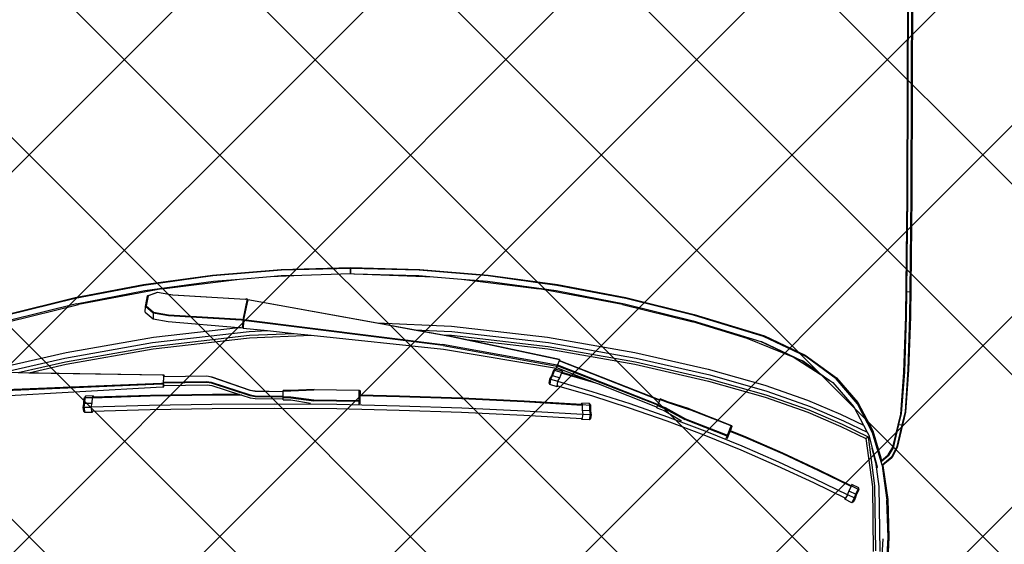
# Model space of a CAD drawing. Units: inches. Extents: x 2167 to 2589, y 1680 to 2489.
# Tile 21 of 38: x 2269 to 2306, y 1796 to 1815. Entities that reach past the tile are written whole.
import ezdxf

# ---------------------------------------------------------------- set-up
doc = ezdxf.new("R2010")
doc.units = ezdxf.units.IN
doc.header["$MEASUREMENT"] = 0
doc.layers.get('0').update_dxf_attribs({"color": 250})
for name, color, linetype, lineweight in [('A-ANNO-DIMS', 2, 'Continuous', 18), ('C-PRKG-VEHS', 8, 'Continuous', 13), ('L-PVMT-PATT', 252, 'Continuous', 13)]:
    doc.layers.add(name, color=color, linetype=linetype, lineweight=lineweight)
doc.layers.add('Edges', color=250, linetype='Continuous')
doc.styles.get("Standard").update_dxf_attribs({"font": 'arial.ttf'})
doc.dimstyles.get("Standard").update_dxf_attribs({"dimtxt": 7, "dimasz": 0.18, "dimexe": 0.18, "dimexo": 0.0625, "dimgap": 0.09, "dimtad": 0, "dimtih": 1, "dimtoh": 1, "dimdec": 1, "dimzin": 0, "dimdsep": 46, "dimlunit": 3, "dimtxsty": 'Standard', "dimcen": 0.09, "dimadec": 0, "dimazin": 0, "dimtfac": 1, "dimtdec": 1, "dimtofl": 0, "dimtmove": 0, "dimatfit": 3, "dimfxl": 1, "dimtolj": 1, "dimtzin": 0, "dimarcsym": 0})

# ---------------------------------------------------------------- blocks, each defined once
blk = doc.blocks.new('Nissan Qashqai pl')
at = {"layer": 'Edges'}
for p, q in [((8.0273, 12.6485), (7.9014, 12.6487)), ((8.0275, 12.6493), (7.902, 12.6495)), ((7.9036, 12.6534), (8.0275, 12.6533)), ((7.904, 12.6547), (8.0276, 12.6545)), ((8.1753, 12.6479), (8.0273, 12.6485)), ((8.0275, 12.6533), (8.1755, 12.6527)), ((8.1754, 12.6487), (8.0275, 12.6493)), ((8.0276, 12.6545), (8.1753, 12.6539)), ((8.1753, 12.6539), (8.3324, 12.6521)), ((8.3318, 12.6462), (8.1753, 12.6479)), ((8.3002, 12.6474), (8.1754, 12.6487)), ((8.1755, 12.6527), (8.3005, 12.6514)), ((8.3005, 12.6514), (8.3002, 12.6474)), ((8.332, 12.6471), (8.3002, 12.6474)), ((8.3005, 12.6514), (8.3324, 12.651)), ((8.4049, 12.6437), (8.3318, 12.6462)), ((8.4042, 12.6447), (8.332, 12.6471)), ((8.3324, 12.6521), (8.4022, 12.6498)), ((8.3324, 12.651), (8.4014, 12.6488)), ((8.4014, 12.6488), (8.4559, 12.6451)), ((8.4022, 12.6498), (8.4571, 12.6459)), ((8.4559, 12.6451), (8.4736, 12.6409)), ((8.4571, 12.6459), (8.5029, 12.635)), ((8.4588, 12.6405), (8.4042, 12.6447)), ((8.4595, 12.6395), (8.4049, 12.6437)), ((8.4729, 12.6372), (8.4588, 12.6405)), ((8.5025, 12.6293), (8.4595, 12.6395)), ((8.4729, 12.6372), (8.4736, 12.6409)), ((8.5032, 12.6301), (8.4729, 12.6372)), ((8.4736, 12.6409), (8.5018, 12.6344)), ((8.5018, 12.6344), (8.5155, 12.6274)), ((8.5029, 12.635), (8.5163, 12.6279)), ((8.5125, 12.6231), (8.5025, 12.6293)), ((8.5132, 12.624), (8.5032, 12.6301)), ((8.5177, 12.617), (8.5125, 12.6231)), ((8.5132, 12.624), (8.5216, 12.6139)), ((8.5155, 12.6274), (8.5258, 12.6151)), ((8.5163, 12.6279), (8.5237, 12.6189)), ((8.5294, 12.6167), (8.5706, 12.6226)), ((8.5304, 12.6157), (8.5715, 12.6215)), ((8.5706, 12.6226), (8.6197, 12.6241)), ((8.6203, 12.6229), (8.5715, 12.6215)), ((8.6197, 12.6241), (8.6683, 12.6215)), ((8.6203, 12.6229), (8.6204, 12.6229)), ((8.6721, 12.6201), (8.6204, 12.6229)), ((8.4814, 12.6029), (8.5166, 12.6135)), ((8.5216, 12.6139), (8.4838, 12.6027)), ((8.5039, 12.6023), (8.528, 12.6088)), ((8.5216, 12.6068), (8.5039, 12.6023)), ((8.5166, 12.6135), (8.5197, 12.6145)), ((8.5197, 12.6145), (8.5177, 12.617)), ((8.5197, 12.6145), (8.5216, 12.6139)), ((8.5258, 12.6151), (8.5216, 12.6139)), ((8.5216, 12.6068), (8.5538, 12.6111)), ((8.5301, 12.609), (8.5216, 12.6068)), ((8.5237, 12.6189), (8.5259, 12.6162)), ((8.5259, 12.6162), (8.5258, 12.6151)), ((8.5258, 12.6151), (8.5304, 12.6157)), ((8.5259, 12.6162), (8.5294, 12.6167)), ((8.5304, 12.6157), (8.5304, 12.6157)), ((8.5531, 12.6055), (8.6375, 12.6066)), ((8.5538, 12.6111), (8.6387, 12.6123)), ((8.622, 12.6161), (8.6699, 12.6132)), ((8.4444, 12.5834), (8.4814, 12.6029)), ((8.4838, 12.6027), (8.4462, 12.5833)), ((8.468, 12.5648), (8.4831, 12.5957)), ((8.4725, 12.563), (8.4889, 12.5969)), ((8.4737, 12.5908), (8.4831, 12.5957)), ((8.4756, 12.5615), (8.4914, 12.5942)), ((8.4831, 12.5957), (8.4867, 12.5977)), ((8.4867, 12.5977), (8.5039, 12.6023)), ((8.4889, 12.5969), (8.5531, 12.6055)), ((8.4914, 12.5942), (8.4889, 12.5969)), ((8.4914, 12.5942), (8.5544, 12.6026)), ((8.5544, 12.6026), (8.6386, 12.6037)), ((8.4122, 12.5558), (8.4444, 12.5834)), ((8.4462, 12.5833), (8.4134, 12.5554)), ((8.4499, 12.5782), (8.4737, 12.5908)), ((8.4594, 12.5611), (8.4737, 12.5908)), ((8.5554, 12.5847), (8.551, 12.5757)), ((8.5529, 12.5751), (8.5572, 12.5841)), ((8.5574, 12.5849), (8.5554, 12.5847)), ((8.5572, 12.5841), (8.5554, 12.5847)), ((8.5639, 12.581), (8.5572, 12.5841)), ((8.5574, 12.5849), (8.5584, 12.5846)), ((8.5582, 12.5845), (8.5574, 12.5849)), ((8.5584, 12.5846), (8.5649, 12.5816)), ((8.5595, 12.572), (8.5639, 12.581)), ((8.5687, 12.5791), (8.5639, 12.581)), ((8.5649, 12.5816), (8.5693, 12.5799)), ((8.4183, 12.5508), (8.4499, 12.5782)), ((8.5527, 12.5749), (8.5323, 12.5332)), ((8.5537, 12.5747), (8.5332, 12.5329)), ((8.5647, 12.57), (8.5441, 12.5279)), ((8.5527, 12.5749), (8.551, 12.5757)), ((8.551, 12.5757), (8.5528, 12.5751)), ((8.5528, 12.5751), (8.5527, 12.5749)), ((8.5528, 12.5751), (8.5529, 12.5751)), ((8.5529, 12.5751), (8.5537, 12.5747)), ((8.5537, 12.5747), (8.5595, 12.572)), ((8.5595, 12.572), (8.5644, 12.5701)), ((8.5644, 12.5701), (8.5687, 12.5791)), ((8.5644, 12.5701), (8.5647, 12.57)), ((8.5647, 12.57), (8.5692, 12.5675)), ((8.5687, 12.5791), (8.5693, 12.5799)), ((8.5749, 12.5757), (8.5687, 12.5791)), ((8.5693, 12.5799), (8.5739, 12.5774)), ((8.5749, 12.5757), (8.5705, 12.5668)), ((8.5739, 12.5774), (8.5749, 12.5757)), ((8.3826, 12.5151), (8.4122, 12.5558)), ((8.4134, 12.5554), (8.3844, 12.5157)), ((8.4411, 12.5178), (8.4594, 12.5611)), ((8.4493, 12.5212), (8.468, 12.5648)), ((8.454, 12.5196), (8.4725, 12.563)), ((8.4571, 12.5184), (8.4756, 12.5615)), ((8.5487, 12.5256), (8.5692, 12.5674)), ((8.5692, 12.5674), (8.5692, 12.5675)), ((8.5692, 12.5675), (8.5705, 12.5668)), ((8.5705, 12.5668), (8.5692, 12.5674)), ((8.4154, 12.5468), (8.3852, 12.4994)), ((8.3901, 12.5113), (8.4154, 12.5468)), ((8.4011, 12.5269), (8.4154, 12.5468)), ((8.4156, 12.547), (8.4154, 12.5468)), ((8.4156, 12.547), (8.4183, 12.5508)), ((8.5323, 12.5332), (8.5103, 12.4859)), ((8.5332, 12.5329), (8.5112, 12.4856)), ((8.4011, 12.5269), (8.3901, 12.5113)), ((8.3904, 12.512), (8.4011, 12.5269)), ((8.4217, 12.4622), (8.4411, 12.5178)), ((8.4296, 12.4651), (8.4493, 12.5212)), ((8.4343, 12.4637), (8.454, 12.5196)), ((8.4375, 12.4627), (8.4571, 12.5184)), ((8.5441, 12.5279), (8.5222, 12.4807)), ((8.5269, 12.4785), (8.5487, 12.5256)), ((8.3573, 12.4618), (8.3826, 12.5151)), ((8.3844, 12.5157), (8.3582, 12.4606)), ((8.3646, 12.4572), (8.39, 12.5111)), ((8.3648, 12.4579), (8.39, 12.5111)), ((8.39, 12.5111), (8.3852, 12.4994)), ((8.39, 12.5111), (8.3901, 12.5113)), ((8.3901, 12.5113), (8.3904, 12.512)), ((8.3852, 12.4994), (8.3608, 12.4393)), ((8.5103, 12.4859), (8.4895, 12.4381)), ((8.5112, 12.4856), (8.4904, 12.4377)), ((8.5222, 12.4807), (8.5014, 12.4329)), ((8.5062, 12.431), (8.5269, 12.4785)), ((8.3296, 12.3703), (8.3573, 12.4618)), ((8.3582, 12.4606), (8.3311, 12.3708)), ((8.3377, 12.3689), (8.3646, 12.4572)), ((8.3646, 12.4572), (8.3648, 12.4579)), ((8.3648, 12.4579), (8.3648, 12.4579)), ((8.4009, 12.3883), (8.4217, 12.4622)), ((8.4084, 12.3907), (8.4296, 12.4651)), ((8.4133, 12.3896), (8.4343, 12.4637)), ((8.4165, 12.3888), (8.4375, 12.4627)), ((8.3608, 12.4393), (8.3392, 12.3684)), ((8.3608, 12.4393), (8.3608, 12.4393)), ((8.4895, 12.4381), (8.4811, 12.4174)), ((8.5014, 12.4329), (8.4817, 12.3847)), ((8.4904, 12.4377), (8.482, 12.4171)), ((8.4866, 12.3829), (8.5062, 12.431)), ((8.4526, 12.3639), (8.4742, 12.4188)), ((8.4747, 12.4185), (8.4532, 12.3636)), ((8.4742, 12.4188), (8.4754, 12.4193)), ((8.4747, 12.4185), (8.4742, 12.4188)), ((8.4754, 12.4193), (8.4747, 12.4185)), ((8.4869, 12.4136), (8.4747, 12.4185)), ((8.4754, 12.4193), (8.4876, 12.4144)), ((8.4791, 12.4183), (8.4754, 12.4193)), ((8.4811, 12.4174), (8.4791, 12.4183)), ((8.482, 12.4171), (8.4811, 12.4174)), ((8.4912, 12.4133), (8.482, 12.4171)), ((8.4869, 12.4136), (8.4876, 12.4144)), ((8.4876, 12.4144), (8.4912, 12.4133)), ((8.4876, 12.4144), (8.4881, 12.4131)), ((8.4654, 12.3587), (8.4869, 12.4136)), ((8.4881, 12.4131), (8.4666, 12.3582)), ((8.4881, 12.4131), (8.4869, 12.4136)), ((8.4914, 12.4121), (8.4881, 12.4131)), ((8.4913, 12.4133), (8.4912, 12.4133)), ((8.4913, 12.4132), (8.4913, 12.4133)), ((8.3792, 12.2926), (8.4009, 12.3883)), ((8.3864, 12.2945), (8.4084, 12.3907)), ((8.3913, 12.2935), (8.4133, 12.3896)), ((8.3945, 12.2929), (8.4165, 12.3888)), ((8.4817, 12.3847), (8.4633, 12.3359)), ((8.4683, 12.3345), (8.4866, 12.3829)), ((8.3076, 12.281), (8.3296, 12.3703)), ((8.3311, 12.3708), (8.3089, 12.2811)), ((8.3157, 12.2795), (8.3377, 12.3689)), ((8.3166, 12.2767), (8.3392, 12.3684)), ((8.4526, 12.3639), (8.4434, 12.3353)), ((8.4439, 12.335), (8.4532, 12.3636)), ((8.4509, 12.3322), (8.4654, 12.3587)), ((8.4521, 12.3317), (8.4666, 12.3582)), ((8.4547, 12.3309), (8.4682, 12.3538)), ((8.3894, 12.1944), (8.4409, 12.3255)), ((8.4415, 12.3252), (8.3899, 12.1941)), ((8.4434, 12.3353), (8.4397, 12.326)), ((8.4403, 12.3257), (8.4397, 12.326)), ((8.4403, 12.3257), (8.4439, 12.335)), ((8.4409, 12.3255), (8.4403, 12.3257)), ((8.4415, 12.3252), (8.4409, 12.3255)), ((8.4467, 12.3231), (8.4415, 12.3252)), ((8.4633, 12.3359), (8.4461, 12.2868)), ((8.4472, 12.3229), (8.4509, 12.3322)), ((8.4484, 12.3224), (8.4521, 12.3317)), ((8.4511, 12.3216), (8.4547, 12.3309)), ((8.4512, 12.2856), (8.4683, 12.3345)), ((8.3951, 12.192), (8.4467, 12.3231)), ((8.4479, 12.3226), (8.3963, 12.1915)), ((8.4209, 12.2475), (8.4502, 12.3219)), ((8.4472, 12.3229), (8.4467, 12.3231)), ((8.4479, 12.3226), (8.4472, 12.3229)), ((8.4484, 12.3224), (8.4479, 12.3226)), ((8.4502, 12.3219), (8.4484, 12.3224)), ((8.4511, 12.3216), (8.4502, 12.3219)), ((8.3593, 12.1791), (8.3792, 12.2926)), ((8.3662, 12.1803), (8.3864, 12.2945)), ((8.3713, 12.1796), (8.3913, 12.2935)), ((8.3745, 12.1792), (8.3945, 12.2929)), ((8.4461, 12.2868), (8.4302, 12.2373)), ((8.4353, 12.2363), (8.4512, 12.2856)), ((8.2905, 12.1918), (8.3076, 12.281)), ((8.3089, 12.2811), (8.2916, 12.1913)), ((8.3166, 12.2767), (8.296, 12.168)), ((8.2985, 12.1901), (8.3157, 12.2795)), ((8.4163, 12.2359), (8.4209, 12.2475)), ((8.4209, 12.2475), (8.4191, 12.2418)), ((8.3986, 12.1908), (8.4163, 12.2359)), ((8.4163, 12.2359), (8.4052, 12.1979)), ((8.4191, 12.2418), (8.4061, 12.1973)), ((8.4302, 12.2373), (8.4171, 12.1926)), ((8.4224, 12.1919), (8.4353, 12.2363)), ((8.4475, 12.2348), (8.4457, 12.2337)), ((8.4475, 12.2348), (8.4484, 12.235)), ((8.4555, 12.2348), (8.4475, 12.2348)), ((8.4484, 12.235), (8.4557, 12.235)), ((8.46, 12.2348), (8.4549, 12.2341)), ((8.4557, 12.235), (8.4603, 12.2357)), ((8.4595, 12.2249), (8.46, 12.2348)), ((8.46, 12.2348), (8.4603, 12.2357)), ((8.4671, 12.2337), (8.46, 12.2348)), ((8.4603, 12.2357), (8.4655, 12.2348)), ((8.4655, 12.2348), (8.4671, 12.2337)), ((8.4471, 12.2238), (8.4425, 12.1485)), ((8.448, 12.2241), (8.4435, 12.1487)), ((8.4457, 12.2337), (8.4452, 12.2238)), ((8.4452, 12.2238), (8.4471, 12.2242)), ((8.4471, 12.2238), (8.4452, 12.2238)), ((8.4476, 12.2341), (8.4457, 12.2337)), ((8.4471, 12.2242), (8.4476, 12.2341)), ((8.4471, 12.2242), (8.4544, 12.2242)), ((8.4471, 12.2239), (8.4471, 12.2238)), ((8.4549, 12.2341), (8.4476, 12.2341)), ((8.4544, 12.2242), (8.4549, 12.2341)), ((8.4544, 12.2242), (8.4595, 12.2249)), ((8.4601, 12.2247), (8.4555, 12.1488)), ((8.4595, 12.2249), (8.4666, 12.2237)), ((8.4607, 12.1481), (8.4652, 12.2237)), ((8.4652, 12.2237), (8.4652, 12.2238)), ((8.4666, 12.2237), (8.4652, 12.2237)), ((8.4671, 12.2337), (8.4666, 12.2237)), ((8.4035, 12.1986), (8.4007, 12.189)), ((8.4023, 12.1879), (8.4052, 12.1975)), ((8.4052, 12.1975), (8.4035, 12.1986)), ((8.4035, 12.1986), (8.4052, 12.1979)), ((8.4052, 12.1979), (8.4052, 12.1978)), ((8.412, 12.195), (8.4052, 12.1975)), ((8.2781, 12.1018), (8.2905, 12.1918)), ((8.2916, 12.1913), (8.2793, 12.1016)), ((8.2862, 12.1008), (8.2985, 12.1901)), ((8.3887, 12.1946), (8.3575, 12.0475)), ((8.3882, 12.1948), (8.3618, 12.07)), ((8.3957, 12.1917), (8.3688, 12.0419)), ((8.3702, 12.0427), (8.3969, 12.1913)), ((8.3746, 12.0435), (8.3995, 12.1905)), ((8.3887, 12.1946), (8.3882, 12.1948)), ((8.3882, 12.1948), (8.3894, 12.1944)), ((8.3894, 12.1944), (8.3887, 12.1946)), ((8.3894, 12.1944), (8.3894, 12.1944)), ((8.3894, 12.1944), (8.3899, 12.1941)), ((8.3899, 12.1941), (8.3951, 12.192)), ((8.3951, 12.192), (8.3963, 12.1915)), ((8.3957, 12.1917), (8.3951, 12.192)), ((8.3969, 12.1913), (8.3957, 12.1917)), ((8.3963, 12.1915), (8.3986, 12.1908)), ((8.3995, 12.1905), (8.3969, 12.1913)), ((8.3995, 12.1905), (8.3986, 12.1908)), ((8.4007, 12.189), (8.4023, 12.1879)), ((8.4007, 12.189), (8.402, 12.1874)), ((8.4028, 12.1868), (8.402, 12.1874)), ((8.402, 12.1874), (8.4027, 12.1871)), ((8.4023, 12.1879), (8.4092, 12.1855)), ((8.4097, 12.1844), (8.4028, 12.1868)), ((8.4092, 12.1855), (8.412, 12.195)), ((8.4092, 12.1855), (8.4139, 12.1829)), ((8.4139, 12.1821), (8.4097, 12.1844)), ((8.4167, 12.1925), (8.412, 12.195)), ((8.4139, 12.1829), (8.4167, 12.1925)), ((8.4139, 12.1829), (8.4209, 12.1819)), ((8.4139, 12.1821), (8.4139, 12.1829)), ((8.4237, 12.1914), (8.4167, 12.1925)), ((8.4237, 12.1914), (8.4209, 12.1819)), ((8.4223, 12.1918), (8.4224, 12.1919)), ((8.4224, 12.1919), (8.4237, 12.1914)), ((8.3448, 12.0536), (8.3593, 12.1791)), ((8.3516, 12.0542), (8.3662, 12.1803)), ((8.3567, 12.0538), (8.3713, 12.1796)), ((8.3618, 12.07), (8.3745, 12.1792)), ((8.4191, 12.1813), (8.4139, 12.1821)), ((8.4209, 12.1819), (8.4191, 12.1813)), ((8.2834, 12.0669), (8.296, 12.168)), ((8.4425, 12.1485), (8.4387, 12.0674)), ((8.4435, 12.1487), (8.4397, 12.0674)), ((8.4555, 12.1488), (8.4517, 12.0674)), ((8.4568, 12.0669), (8.4607, 12.1481)), ((8.2708, 12.0123), (8.2781, 12.1018)), ((8.2793, 12.1016), (8.2719, 12.0118)), ((8.2834, 12.0669), (8.2862, 12.1008)), ((8.3618, 12.07), (8.3574, 12.0489)), ((8.4387, 12.0674), (8.4359, 11.9861)), ((8.4397, 12.0674), (8.4369, 11.9861)), ((8.4517, 12.0674), (8.4489, 11.9858)), ((8.2804, 12.0305), (8.2834, 12.0669)), ((8.4541, 11.9857), (8.4568, 12.0669)), ((8.3575, 12.0475), (8.3104, 11.7881)), ((8.336, 11.7828), (8.3688, 12.0419)), ((8.3702, 12.0427), (8.3374, 11.7826)), ((8.3406, 11.9567), (8.3448, 12.0536)), ((8.3495, 12.0053), (8.3516, 12.0542)), ((8.3495, 12.0053), (8.3562, 12.0421)), ((8.3562, 12.0421), (8.3567, 12.0538)), ((8.3562, 12.0421), (8.3574, 12.0489)), ((8.3565, 11.8707), (8.3746, 12.0435)), ((8.2765, 11.9273), (8.2804, 12.0305)), ((8.2788, 12.0114), (8.2804, 12.0305)), ((8.2682, 11.9221), (8.2708, 12.0123)), ((8.2719, 12.0118), (8.2695, 11.9221)), ((8.2765, 11.9273), (8.2788, 12.0114)), ((8.3406, 11.9567), (8.3495, 12.0053)), ((8.4359, 11.9861), (8.4348, 11.9346)), ((8.4369, 11.9861), (8.4358, 11.9346)), ((8.4489, 11.9858), (8.4471, 11.9043)), ((8.4523, 11.9043), (8.4541, 11.9857)), ((8.31, 11.7882), (8.3406, 11.9567)), ((8.2763, 11.9223), (8.2764, 11.9263)), ((8.2764, 11.9263), (8.2765, 11.9273)), ((8.4272, 11.8746), (8.4281, 11.9336)), ((8.4287, 11.9335), (8.4278, 11.8745)), ((8.4281, 11.9336), (8.429, 11.9345)), ((8.4281, 11.9336), (8.4287, 11.9336)), ((8.4287, 11.9335), (8.4281, 11.9336)), ((8.429, 11.9345), (8.4287, 11.9336)), ((8.4287, 11.9336), (8.4287, 11.9335)), ((8.4418, 11.9332), (8.4287, 11.9335)), ((8.4328, 11.9347), (8.429, 11.9345)), ((8.429, 11.9345), (8.4326, 11.9345)), ((8.4328, 11.9347), (8.4326, 11.9345)), ((8.4326, 11.9345), (8.4348, 11.9344)), ((8.4348, 11.9346), (8.4328, 11.9347)), ((8.4348, 11.9346), (8.4348, 11.9344)), ((8.4358, 11.9346), (8.4348, 11.9346)), ((8.4348, 11.9344), (8.4358, 11.9344)), ((8.4358, 11.9346), (8.4358, 11.9344)), ((8.4459, 11.9344), (8.4358, 11.9346)), ((8.4358, 11.9344), (8.4422, 11.9342)), ((8.441, 11.8742), (8.4418, 11.9332)), ((8.4418, 11.9332), (8.4422, 11.9342)), ((8.4431, 11.9332), (8.4418, 11.9332)), ((8.4422, 11.9342), (8.4459, 11.9344)), ((8.4422, 11.9342), (8.4431, 11.9332)), ((8.4431, 11.9332), (8.4422, 11.8742)), ((8.4464, 11.9334), (8.4431, 11.9332)), ((8.4459, 11.9344), (8.4459, 11.9344)), ((8.2708, 11.8319), (8.2682, 11.9221)), ((8.2763, 11.9223), (8.2695, 11.9221)), ((8.2695, 11.9221), (8.2763, 11.9219)), ((8.2695, 11.9221), (8.2719, 11.8323)), ((8.2763, 11.9219), (8.2763, 11.9223)), ((8.2781, 11.8585), (8.2763, 11.9219)), ((8.4471, 11.9043), (8.4464, 11.8227)), ((8.4516, 11.823), (8.4523, 11.9043)), ((8.3542, 11.8485), (8.3565, 11.8707)), ((8.3599, 11.7906), (8.3565, 11.8707)), ((8.4272, 11.8746), (8.4286, 11.8445)), ((8.4292, 11.8445), (8.4278, 11.8745)), ((8.4368, 11.8443), (8.441, 11.8742)), ((8.438, 11.8443), (8.4422, 11.8742)), ((8.4408, 11.8444), (8.4452, 11.8698)), ((8.28, 11.818), (8.2781, 11.8585)), ((8.2788, 11.8327), (8.2781, 11.8585)), ((8.2789, 11.8319), (8.2781, 11.8585)), ((8.3505, 11.8139), (8.3542, 11.8485)), ((8.3567, 11.7903), (8.3542, 11.8485)), ((8.4286, 11.8445), (8.4285, 11.8345)), ((8.4291, 11.8345), (8.4292, 11.8445)), ((8.4366, 11.8345), (8.4368, 11.8443)), ((8.4379, 11.8345), (8.438, 11.8443)), ((8.4406, 11.8344), (8.4408, 11.8444)), ((8.2781, 11.7423), (8.2708, 11.8319)), ((8.2719, 11.8323), (8.2793, 11.7426)), ((8.2789, 11.8319), (8.2788, 11.8327)), ((8.28, 11.818), (8.2789, 11.8319)), ((8.4291, 11.8345), (8.4285, 11.8345)), ((8.4298, 11.8345), (8.4291, 11.8345)), ((8.4292, 11.7978), (8.4298, 11.8345)), ((8.4304, 11.8345), (8.4298, 11.7978)), ((8.4304, 11.8345), (8.4298, 11.8345)), ((8.436, 11.8344), (8.4304, 11.8345)), ((8.4355, 11.7977), (8.436, 11.8344)), ((8.4366, 11.8343), (8.436, 11.8344)), ((8.4366, 11.8345), (8.4379, 11.8345)), ((8.4366, 11.8344), (8.4366, 11.8345)), ((8.4373, 11.8344), (8.4366, 11.8344)), ((8.4373, 11.8344), (8.4366, 11.8343)), ((8.4366, 11.8343), (8.4366, 11.8344)), ((8.4373, 11.8344), (8.4367, 11.7977)), ((8.4379, 11.8344), (8.4373, 11.8344)), ((8.4379, 11.8343), (8.4373, 11.8344)), ((8.4379, 11.8344), (8.4379, 11.8345)), ((8.4397, 11.8344), (8.4379, 11.8343)), ((8.4379, 11.8343), (8.4379, 11.8344)), ((8.4391, 11.7978), (8.4397, 11.8344)), ((8.4406, 11.8344), (8.4397, 11.8344)), ((8.2834, 11.7773), (8.28, 11.818)), ((8.3472, 11.7821), (8.3505, 11.8139)), ((8.3516, 11.79), (8.3505, 11.8139)), ((8.4464, 11.8227), (8.4468, 11.7413)), ((8.452, 11.7418), (8.4516, 11.823)), ((8.4281, 11.7914), (8.4292, 11.7978)), ((8.4298, 11.7978), (8.4287, 11.7914)), ((8.4344, 11.7912), (8.4355, 11.7977)), ((8.4367, 11.7977), (8.4357, 11.7912)), ((8.4381, 11.7914), (8.4391, 11.7978)), ((8.3038, 11.6903), (8.3095, 11.7853)), ((8.3099, 11.7851), (8.3042, 11.6901)), ((8.3092, 11.7863), (8.3093, 11.7873)), ((8.3092, 11.7863), (8.3099, 11.7851)), ((8.3095, 11.7853), (8.3092, 11.7863)), ((8.3093, 11.7873), (8.3367, 11.7816)), ((8.3159, 11.7869), (8.3093, 11.7873)), ((8.31, 11.7882), (8.3104, 11.7881)), ((8.3104, 11.7881), (8.3159, 11.7869)), ((8.3159, 11.7869), (8.336, 11.7828)), ((8.3662, 11.6639), (8.3516, 11.79)), ((8.3713, 11.6645), (8.3567, 11.7903)), ((8.3745, 11.665), (8.3599, 11.7906)), ((8.4107, 11.7411), (8.4281, 11.7914)), ((8.4287, 11.7914), (8.4111, 11.741)), ((8.4179, 11.7406), (8.4344, 11.7912)), ((8.4357, 11.7912), (8.4193, 11.7407)), ((8.4347, 11.7805), (8.4381, 11.7914)), ((8.296, 11.6762), (8.2834, 11.7773)), ((8.2862, 11.7434), (8.2834, 11.7773)), ((8.3298, 11.6848), (8.3355, 11.7798)), ((8.3369, 11.7796), (8.3312, 11.6846)), ((8.3355, 11.7798), (8.3366, 11.7806)), ((8.336, 11.7828), (8.3374, 11.7826)), ((8.3367, 11.7816), (8.3366, 11.7806)), ((8.3366, 11.7806), (8.3369, 11.7796)), ((8.3367, 11.7816), (8.347, 11.7811)), ((8.3374, 11.7826), (8.3406, 11.7824)), ((8.3385, 11.6842), (8.3464, 11.7761)), ((8.3458, 11.7813), (8.3406, 11.7824)), ((8.3406, 11.7824), (8.3457, 11.7821)), ((8.3458, 11.7813), (8.3457, 11.7821)), ((8.3457, 11.7821), (8.3472, 11.7821)), ((8.347, 11.7811), (8.3458, 11.7813)), ((8.3464, 11.7761), (8.3467, 11.7791)), ((8.3593, 11.6651), (8.3464, 11.7761)), ((8.3467, 11.7791), (8.347, 11.7811)), ((8.4222, 11.7413), (8.4337, 11.7775)), ((8.4337, 11.7775), (8.4347, 11.7805)), ((8.4337, 11.7775), (8.4339, 11.7423)), ((8.4347, 11.7805), (8.4348, 11.7421)), ((8.2905, 11.6524), (8.2781, 11.7423)), ((8.2793, 11.7426), (8.2916, 11.6528)), ((8.2985, 11.654), (8.2862, 11.7434)), ((8.4097, 11.7348), (8.4107, 11.7411)), ((8.4104, 11.6791), (8.4097, 11.7348)), ((8.4111, 11.741), (8.41, 11.7346)), ((8.41, 11.7346), (8.4108, 11.6791)), ((8.417, 11.7342), (8.4179, 11.7406)), ((8.4177, 11.678), (8.417, 11.7342)), ((8.4193, 11.7407), (8.4183, 11.7343)), ((8.4183, 11.7343), (8.4191, 11.678)), ((8.4213, 11.735), (8.4222, 11.7413)), ((8.4221, 11.6787), (8.4213, 11.735)), ((8.4339, 11.7423), (8.4353, 11.6613)), ((8.4348, 11.7421), (8.4362, 11.661)), ((8.4468, 11.7413), (8.4482, 11.66)), ((8.4534, 11.6608), (8.452, 11.7418)), ((8.3005, 11.6706), (8.3038, 11.6903)), ((8.3042, 11.6901), (8.3009, 11.6704)), ((8.3264, 11.6652), (8.3298, 11.6848)), ((8.3312, 11.6846), (8.3278, 11.665)), ((8.3352, 11.6646), (8.3385, 11.6842)), ((8.296, 11.6762), (8.3166, 11.5675)), ((8.3053, 11.6574), (8.3005, 11.6706)), ((8.3009, 11.6704), (8.3054, 11.6583)), ((8.4086, 11.6764), (8.4045, 11.4011)), ((8.4056, 11.5028), (8.4082, 11.6766)), ((8.4082, 11.6785), (8.4104, 11.6791)), ((8.4082, 11.6785), (8.4086, 11.6784)), ((8.4082, 11.6766), (8.4082, 11.6785)), ((8.4086, 11.6784), (8.4086, 11.6764)), ((8.4086, 11.6784), (8.4117, 11.6782)), ((8.4104, 11.6791), (8.4108, 11.6791)), ((8.4104, 11.6786), (8.4104, 11.6791)), ((8.4108, 11.6786), (8.4104, 11.6786)), ((8.4104, 11.6786), (8.4108, 11.6784)), ((8.4108, 11.6791), (8.4108, 11.6786)), ((8.4108, 11.6786), (8.4108, 11.6784)), ((8.4108, 11.6784), (8.4117, 11.6783)), ((8.4117, 11.6783), (8.4117, 11.6782)), ((8.4117, 11.6783), (8.4177, 11.678)), ((8.4117, 11.6782), (8.419, 11.6778)), ((8.4177, 11.678), (8.4191, 11.678)), ((8.419, 11.6778), (8.4203, 11.6778)), ((8.419, 11.6758), (8.419, 11.6778)), ((8.4305, 11.3996), (8.419, 11.6758)), ((8.4191, 11.678), (8.4221, 11.6787)), ((8.4238, 11.6786), (8.4203, 11.6778)), ((8.4203, 11.6778), (8.4204, 11.6758)), ((8.4204, 11.6758), (8.4319, 11.3996)), ((8.4238, 11.6786), (8.4221, 11.6787)), ((8.4238, 11.6766), (8.4238, 11.6786)), ((8.4394, 11.4014), (8.4238, 11.6766)), ((8.3054, 11.6583), (8.3053, 11.6574)), ((8.319, 11.6546), (8.3053, 11.6574)), ((8.3054, 11.6583), (8.3182, 11.6557)), ((8.3182, 11.6557), (8.3264, 11.6652)), ((8.3278, 11.665), (8.319, 11.6546)), ((8.3264, 11.6542), (8.3352, 11.6646)), ((8.3278, 11.665), (8.3352, 11.6646)), ((8.3792, 11.5515), (8.3593, 11.6651)), ((8.3864, 11.5497), (8.3662, 11.6639)), ((8.3913, 11.5506), (8.3713, 11.6645)), ((8.3945, 11.5513), (8.3745, 11.665)), ((8.4353, 11.6613), (8.4375, 11.5863)), ((8.4362, 11.661), (8.4385, 11.5858)), ((8.4482, 11.66), (8.4505, 11.5843)), ((8.4557, 11.5855), (8.4534, 11.6608)), ((8.3076, 11.5631), (8.2905, 11.6524)), ((8.2916, 11.6528), (8.3089, 11.5631)), ((8.3157, 11.5647), (8.2985, 11.654)), ((8.319, 11.6546), (8.3182, 11.6557)), ((8.3264, 11.6542), (8.319, 11.6546)), ((8.4377, 11.5857), (8.4357, 11.5864)), ((8.4357, 11.5864), (8.4359, 11.5765)), ((8.4357, 11.5864), (8.4375, 11.5863)), ((8.4375, 11.5863), (8.4375, 11.5862)), ((8.4379, 11.5758), (8.4377, 11.5857)), ((8.445, 11.5853), (8.4377, 11.5857)), ((8.4452, 11.5754), (8.445, 11.5853)), ((8.4503, 11.5841), (8.445, 11.5853)), ((8.4572, 11.5854), (8.4503, 11.5841)), ((8.4505, 11.5742), (8.4503, 11.5841)), ((8.4557, 11.5855), (8.4572, 11.5854)), ((8.4557, 11.5853), (8.4557, 11.5855)), ((8.4572, 11.5854), (8.4574, 11.5755)), ((8.3392, 11.4758), (8.3166, 11.5675)), ((8.4359, 11.5765), (8.4379, 11.5758)), ((8.4359, 11.5765), (8.4377, 11.5753)), ((8.4387, 11.5749), (8.4377, 11.5753)), ((8.4379, 11.5758), (8.4452, 11.5754)), ((8.4384, 11.5752), (8.4457, 11.5749)), ((8.446, 11.5746), (8.4387, 11.5749)), ((8.4452, 11.5754), (8.4505, 11.5742)), ((8.4507, 11.5734), (8.446, 11.5746)), ((8.4505, 11.5742), (8.4574, 11.5755)), ((8.4507, 11.5734), (8.4505, 11.5742)), ((8.4559, 11.5744), (8.4507, 11.5734)), ((8.4574, 11.5755), (8.4559, 11.5744)), ((8.3296, 11.4739), (8.3076, 11.5631)), ((8.3089, 11.5631), (8.3311, 11.4733)), ((8.3157, 11.5647), (8.3377, 11.4753)), ((8.4009, 11.4559), (8.3792, 11.5515)), ((8.4051, 11.4678), (8.3864, 11.5497)), ((8.4054, 11.4887), (8.3913, 11.5506)), ((8.4056, 11.5028), (8.3945, 11.5513)), ((8.4054, 11.4887), (8.4056, 11.5028))]:
    blk.add_line(p, q, dxfattribs=at)
blk = doc.blocks.new('car')
blk.add_blockref('Nissan Qashqai pl', (-9.7433, -11.9151))
blk = doc.blocks.new('carr')
blk.add_blockref('car', (0.5124, -0.007))
blk = doc.blocks.new('*D45')
at = {"layer": 'A-ANNO-DIMS', "color": 0, "lineweight": -2, "transparency": 16777216}
for p, q in [((2251.156, 1833.955), (2232.359, 1833.955)), ((2232.539, 1833.775), (2232.539, 1775.399)), ((2232.539, 1709.605), (2232.539, 1767.981)), ((2251.156, 1709.425), (2232.359, 1709.425))]:
    blk.add_line(p, q, dxfattribs=at)
at = {"layer": 'A-ANNO-DIMS', "color": 0, "transparency": 16777216}
for points in [[(2232.509, 1833.775), (2232.569, 1833.775), (2232.539, 1833.955)], [(2232.509, 1709.605), (2232.569, 1709.605), (2232.539, 1709.425)]]:
    blk.add_solid(points, dxfattribs=at)
at = {"layer": 'Defpoints', "color": 0, "transparency": 16777216}
for p in [(2251.218, 1833.955), (2232.539, 1709.425), (2251.218, 1709.425)]:
    blk.add_point(p, dxfattribs=at)
at = {"layer": 'A-ANNO-DIMS', "color": 0, "transparency": 16777216, "insert": (2232.539, 1771.69), "char_height": 7, "attachment_point": 5}
blk.add_mtext('\\A1;CAR 10\'-4 1/2" TYP.', dxfattribs=at)

msp = doc.modelspace()

# ---------------------------------------------------------------- hatches: boundary and pattern name
at = {"layer": 'L-PVMT-PATT'}
h = msp.add_hatch(dxfattribs=at)
h.set_pattern_fill('ANSI37', color=256, scale=40)
h.paths.add_polyline_path([(2417.548, 1783.695), (2417.548, 1846.042), (2239.361, 1846.042), (2239.361, 1687.695), (2369.843, 1687.695), (2369.843, 1696.695), (2375.607, 1696.695), (2416.107, 1696.695), (2417.548, 1696.695)])

# ---------------------------------------------------------------- block references
at = {"layer": 'C-PRKG-VEHS', "xscale": 28.42784210623918, "yscale": 28.42784210623918, "zscale": 28.42784210623918, "rotation": 270}
msp.add_blockref('carr', (2281.736, 1778.659), dxfattribs=at)

# ---------------------------------------------------------------- dimensions: what is measured, and where the dimension line sits
at = {"layer": 'A-ANNO-DIMS'}
dim = msp.add_linear_dim(base=(2232.539, 1709.425), p1=(2251.218, 1833.955), p2=(2251.218, 1709.425), angle=270, text='CAR <> TYP.', dimstyle='Standard', override={"dimdec": 1, "dimlfac": 1, "dimrnd": 0, "dimzin": 1, "dimdsep": 46, "dimlunit": 4, "dimfrac": 2}, dxfattribs=at)
dim.commit()
dim.dimension.update_dxf_attribs({"geometry": '*D45', "text_midpoint": (2232.539, 1771.69)})

doc.saveas('drawing.dxf')
